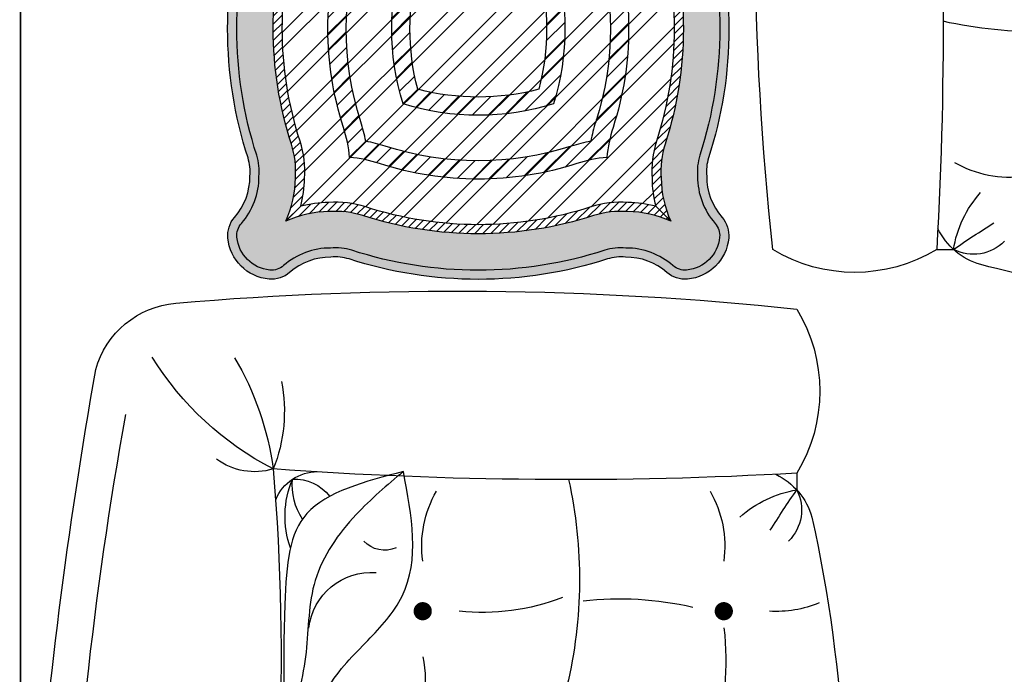
# Model space of a CAD drawing. Units: inches. Extents: x 844 to 2234, y 346 to 1084.
# Tile 63 of 93: x 1843.09 to 1860.31, y 712.91 to 724.36. Entities that reach past the tile are written whole.
import ezdxf

# ---------------------------------------------------------------- set-up
doc = ezdxf.new("R2010")
doc.units = ezdxf.units.IN
doc.header["$MEASUREMENT"] = 0
doc.layers.add('A-WALL', color=7, linetype='Continuous', lineweight=35)
doc.layers.add('furniture', color=8, linetype='Continuous', lineweight=18)
for name, color, linetype in [('RA-AP-01$0$FURN', 3, 'Continuous'), ('RA-AP-01$0$steel', 193, 'Continuous'), ('RA-AP-01$0$WOOD', 64, 'Continuous')]:
    doc.layers.add(name, color=color, linetype=linetype)
pattern_1 = [(45, (0, 1.362436106329781), (-0.0088388347648318, 0.0088388347648318), [])]
pattern_2 = [(45, (0, 1.362436106329781), (-0.0044194173824159, 0.0044194173824159), [])]

# ---------------------------------------------------------------- blocks, each defined once
blk = doc.blocks.new('A$C2FCF5309')
at = {"layer": 'RA-AP-01$0$FURN'}
h = blk.add_hatch(dxfattribs=at)
h.set_pattern_fill('ANSI31', color=256, scale=0.1, style=0)
h.set_pattern_definition(pattern_1)
h.paths.add_polyline_path([(5.038683893313746, -5.169250834004607, -0.1583983521602212), (5.038683893312098, -5.373464580902012, 0.0306258898943267), (5.033304057242972, -5.394827569605182, 0.0306258898948892), (5.01194106853941, -5.40020740567441, -0.1028142994996694), (4.878286182323899, -5.414871334512708), (4.863600873530158, -5.43331743520547, 0.1120482678681049), (5.018059823131753, -5.419248541734471, -0.052642197802937), (5.050972078299936, -5.412495590662115, -0.0526421977994963), (5.057725029371615, -5.379583335496025, 0.1583028414702701), (5.057725029372958, -5.163132079409654, -0.052642197806903), (5.050972078299777, -5.130219824239078, -0.0526421977995126), (5.018059823133679, -5.123466873167369, 0.0215995840215353), (4.988903013548211, -5.115372132362452), (4.975007495303644, -5.132826183367946, -0.0289147572844802), (5.011941068537408, -5.142508009226167, 0.0306258898976746), (5.033304057242868, -5.147887845296027, 0.0306258899022411)])
h.paths.add_polyline_path([(4.975007495303645, -5.132826183367946), (4.988903013548211, -5.115372132362452, 0.1362374241599938), (4.801608567045604, -5.12346687316654, -0.0526421978036853), (4.768696311876971, -5.130219824239102, -0.05264219780204), (4.761943360804856, -5.163132079406747, 0.1583028414743723), (4.761943360806116, -5.379583335498449, -0.0526421977955461), (4.768696311877141, -5.412495590662114, -0.0526421978073986), (4.801608567048022, -5.419248541735437, 0.0454484293938888), (4.863600873530158, -5.43331743520547), (4.878286182323899, -5.414871334512708, -0.0546933379798044), (4.80772732164382, -5.40020740567649, 0.030625889903973), (4.786364332934043, -5.394827569605216, 0.0306258898932853), (4.780984496865101, -5.373464580902791, -0.1583983521638281), (4.780984496864308, -5.169250834000963, 0.03062588989692), (4.786364332933943, -5.147887845296004, 0.0306258898946324), (4.807727321637318, -5.142508009226805, -0.1288932573266927)])
h.paths.add_polyline_path([(4.843422214712861, -5.204945727074827, -0.0783685831716868), (4.924134454130224, -5.196727409635105), (4.939146578618322, -5.177870798323143, 0.1012675676854134), (4.827248748758957, -5.188772261120899, 0.1253648873081696), (4.820394258584192, -5.327034652050361), (4.837127701354095, -5.306015906404253, -0.0981593964869636)], flags=17)
h.paths.add_polyline_path([(4.843422214712824, -5.337769687826355, -0.0311091841722656), (4.837127701354095, -5.306015906404253), (4.820394258584193, -5.32703465205036, 0.0247727657431944), (4.827248748758908, -5.353943153780261, 0.0812754385032542), (4.916962478476905, -5.36629034358622), (4.933684093813825, -5.345286454285511, -0.0876255421014372)], flags=17)
h.paths.add_polyline_path([(4.992419641418037, -5.353943153780226, 0.1506053783834298), (4.992419641417933, -5.188772261120954, 0.0485966419124224), (4.939146578618321, -5.177870798323143), (4.924134454130224, -5.196727409635105, -0.0507799419579301), (4.976246175464031, -5.204945727074882, -0.1296645318906876), (4.97624617546411, -5.337769687826316, -0.0415667119298777), (4.933684093813825, -5.345286454285511), (4.916962478476905, -5.36629034358622, 0.0684915676023693)], flags=17)
h = blk.add_hatch(dxfattribs=at)
h.set_pattern_fill('ANSI31', color=256, scale=0.1, style=0)
h.set_pattern_definition(pattern_1)
h.paths.add_polyline_path([(5.038683893313746, -5.169250834004607, -0.1583983521602212), (5.038683893312098, -5.373464580902012, 0.0306258898943267), (5.033304057242972, -5.394827569605182, 0.0306258898948892), (5.01194106853941, -5.40020740567441, -0.1028142994996694), (4.878286182323899, -5.414871334512708), (4.863600873530158, -5.43331743520547, 0.1120482678681049), (5.018059823131753, -5.419248541734471, -0.052642197802937), (5.050972078299936, -5.412495590662115, -0.0526421977994963), (5.057725029371615, -5.379583335496025, 0.1583028414702701), (5.057725029372958, -5.163132079409654, -0.052642197806903), (5.050972078299777, -5.130219824239078, -0.0526421977995126), (5.018059823133679, -5.123466873167369, 0.0215995840215353), (4.988903013548211, -5.115372132362452), (4.975007495303644, -5.132826183367946, -0.0289147572844802), (5.011941068537408, -5.142508009226167, 0.0306258898976746), (5.033304057242868, -5.147887845296027, 0.0306258899022411)])
h.paths.add_polyline_path([(4.975007495303645, -5.132826183367946), (4.988903013548211, -5.115372132362452, 0.1362374241599938), (4.801608567045604, -5.12346687316654, -0.0526421978036853), (4.768696311876971, -5.130219824239102, -0.05264219780204), (4.761943360804856, -5.163132079406747, 0.1583028414743723), (4.761943360806116, -5.379583335498449, -0.0526421977955461), (4.768696311877141, -5.412495590662114, -0.0526421978073986), (4.801608567048022, -5.419248541735437, 0.0454484293938888), (4.863600873530158, -5.43331743520547), (4.878286182323899, -5.414871334512708, -0.0546933379798044), (4.80772732164382, -5.40020740567649, 0.030625889903973), (4.786364332934043, -5.394827569605216, 0.0306258898932853), (4.780984496865101, -5.373464580902791, -0.1583983521638281), (4.780984496864308, -5.169250834000963, 0.03062588989692), (4.786364332933943, -5.147887845296004, 0.0306258898946324), (4.807727321637318, -5.142508009226805, -0.1288932573266927)])
h.paths.add_polyline_path([(4.843422214712861, -5.204945727074827, -0.0783685831716868), (4.924134454130224, -5.196727409635105), (4.939146578618322, -5.177870798323143, 0.1012675676854134), (4.827248748758957, -5.188772261120899, 0.1253648873081696), (4.820394258584192, -5.327034652050361), (4.837127701354095, -5.306015906404253, -0.0981593964869636)], flags=17)
h.paths.add_polyline_path([(4.843422214712824, -5.337769687826355, -0.0311091841722656), (4.837127701354095, -5.306015906404253), (4.820394258584193, -5.32703465205036, 0.0247727657431944), (4.827248748758908, -5.353943153780261, 0.0812754385032542), (4.916962478476905, -5.36629034358622), (4.933684093813825, -5.345286454285511, -0.0876255421014372)], flags=17)
h.paths.add_polyline_path([(4.992419641418037, -5.353943153780226, 0.1506053783834298), (4.992419641417933, -5.188772261120954, 0.0485966419124224), (4.939146578618321, -5.177870798323143), (4.924134454130224, -5.196727409635105, -0.0507799419579301), (4.976246175464031, -5.204945727074882, -0.1296645318906876), (4.97624617546411, -5.337769687826316, -0.0415667119298777), (4.933684093813825, -5.345286454285511), (4.916962478476905, -5.36629034358622, 0.0684915676023693)], flags=17)
at = {"layer": 'RA-AP-01$0$WOOD'}
h = blk.add_hatch(color=256, dxfattribs=at)
edge = h.paths.add_edge_path()
edge.add_arc((4.683001772622394, -5.026441828662609), 0.0299999999999998, 48.77105092035535, 95.25687599427813)
edge.add_arc((4.684834195088484, -5.046357707450686), 0.0499999999998897, 95.25687599443106, 174.7431240064049)
edge.add_arc((4.664918316300367, -5.044525284985046), 0.0300000000000005, 174.7431240062535, 221.2289490796905)
edge.add_arc((4.591236830209155, -5.109094338216345), 0.0679700159630267, -0.5333070513215148, 41.228949079691915, ccw=False)
edge.add_arc((4.609451302807284, -5.114694777173187), 0.0500000000000008, -17.3556839752095, 5.7020707654044145, ccw=False)
edge.add_arc((5.095208119646659, -5.271357707450659), 0.4603971832811796, 162.0683908477609, 197.9316091523306)
edge.add_arc((4.609451302807533, -5.428020637728902), 0.0500000000000006, -5.702070765320514, 17.355683975293914, ccw=False)
edge.add_arc((4.591236830209412, -5.433621076685779), 0.0679700159630261, -41.228949079600625, 0.5333070514128053, ccw=False)
edge.add_arc((4.664918316300727, -5.498190129916959), 0.0299999999999995, 138.7710509204022, 185.256875994324)
edge.add_arc((4.684834195088642, -5.496357707450695), 0.0499999999997451, 185.2568759946742, 264.74312400432)
edge.add_arc((4.683001772622394, -5.516273586238612), 0.03, 264.743124003969, 311.2289490796446)
edge.add_arc((4.747570825853633, -5.589955072329876), 0.0679700159630271, 89.4666929486321, 131.2289490796457, ccw=False)
edge.add_arc((4.753171264810493, -5.57174059973175), 0.0500000000000015, 72.64431602474701, 95.70207076536133, ccw=False)
edge.add_arc((4.909834195088355, -5.085983782892503), 0.4603971832811774, 252.0683908477147, 287.9316091522845)
edge.add_arc((5.06649712536621, -5.57174059973175), 0.0499999999999999, 84.29792923463953, 107.35568397525361, ccw=False)
edge.add_arc((5.072097564323069, -5.589955072329877), 0.0679700159630274, 48.771050920354185, 90.5333070513679, ccw=False)
edge.add_arc((5.136666617554309, -5.516273586238614), 0.0299999999999997, 228.771050920353, 275.2568759942969)
edge.add_arc((5.134834195088338, -5.496357707450417), 0.0499999999999982, 275.2568759942949, 354.7431240057633)
edge.add_arc((5.154750073876535, -5.498190129916372), 0.0299999999999999, 354.7431240057662, 401.2289490796891)
edge.add_arc((5.228431559967749, -5.433621076685074), 0.0679700159630274, 179.4666929486771, 221.2289490796903, ccw=False)
edge.add_arc((5.210217087369615, -5.428020637728227), 0.0499999999999976, 162.6443160247947, 185.7020707654089, ccw=False)
edge.add_arc((4.724460270530244, -5.271357707450757), 0.4603971832811793, 342.0683908477607, 377.9316091523305)
edge.add_arc((5.210217087369368, -5.114694777172509), 0.0500000000000019, 174.2979292346878, 197.355683975302, ccw=False)
edge.add_arc((5.228431559967489, -5.109094338215639), 0.0679700159630279, 138.7710509203993, 180.5333070514128, ccw=False)
edge.add_arc((5.154750073876174, -5.044525284984457), 0.0300000000000001, 318.771050920401, 365.2568759954636)
edge.add_arc((5.13483419508816, -5.046357707450624), 0.0499999999998349, 5.256875995237118, 84.74312400549572)
edge.add_arc((5.136666617554308, -5.026441828662608), 0.0299999999999994, 84.74312400572185, 131.2289490796446)
edge.add_arc((5.072097564323072, -4.952760342571343), 0.0679700159630261, 269.4666929486298, 311.22894907964354, ccw=False)
edge.add_arc((5.066497125366206, -4.97097481516947), 0.0499999999999992, 252.64431602475162, 275.70207076536565, ccw=False)
edge.add_arc((4.909834195088355, -5.456731632008717), 0.4603971832811764, 72.06839084771546, 107.9316091522853)
edge.add_arc((4.753171264810493, -4.970974815169471), 0.0500000000000016, 264.2979292346387, 287.355683975253, ccw=False)
edge.add_arc((4.747570825853633, -4.952760342571346), 0.0679700159630274, 228.7710509203543, 270.5333070513679, ccw=False)
edge = h.paths.add_edge_path(flags=16)
edge.add_arc((4.683001772622395, -5.026441828662608), 0.019999999999999, 48.7710509203555, 95.2568759942793)
edge.add_arc((4.684834195088469, -5.046357707450671), 0.0399999999998731, 95.2568759944489, 174.7431240064248)
edge.add_arc((4.664918316300404, -5.044525284985035), 0.020000000000036, 174.7431240062186, 221.2289490796461)
edge.add_arc((4.591236830209151, -5.109094338216346), 0.0779700159630296, -0.13764630038667747, 41.228949079689585, ccw=False)
edge.add_arc((4.609451302807307, -5.11469477717304), 0.060000000000024, -17.406127045137907, 5.176192161068002, ccw=False)
edge.add_arc((5.09520811964665, -5.271357707450659), 0.4503971832811708, 162.0623235129628, 197.9376764869162)
edge.add_arc((4.609451302807532, -5.428020637728943), 0.0599999999999982, -5.176192160466428, 17.406127046715312, ccw=False)
edge.add_arc((4.591236830209414, -5.433621076685778), 0.0779700159630257, -41.2289490796029, 0.13764630095249686, ccw=False)
edge.add_arc((4.664918316300731, -5.498190129916961), 0.0200000000000047, 138.7710509204103, 185.2568759943212)
edge.add_arc((4.684834195088606, -5.496357707450731), 0.0399999999997066, 185.2568759947174, 264.7431240043665)
edge.add_arc((4.683001772622369, -5.516273586238541), 0.020000000000069, 264.7431240038842, 311.2289490795622)
edge.add_arc((4.747570825853635, -5.589955072329884), 0.0779700159630344, 89.8623536987642, 131.2289490796432, ccw=False)
edge.add_arc((4.753171264810603, -5.571740599731771), 0.0599999999999895, 72.5938729544394, 95.1761921602253, ccw=False)
edge.add_arc((4.909834195088365, -5.085983782892505), 0.4503971832811724, 252.0623235129989, 287.9376764870498)
edge.add_arc((5.066497125366216, -5.571740599731755), 0.0600000000000047, 84.8238078399923, 107.40612704528041, ccw=False)
edge.add_arc((5.072097564322998, -5.589955072329853), 0.077970015963056, 48.771050920303594, 90.13764630126451, ccw=False)
edge.add_arc((5.136666617554307, -5.516273586238622), 0.0199999999999931, 228.771050920344, 275.2568759943037)
edge.add_arc((5.134834195088338, -5.496357707450416), 0.0400000000000004, 275.2568759942928, 354.7431240057607)
edge.add_arc((5.154750073876533, -5.498190129916375), 0.0200000000000037, 354.7431240057783, 401.2289490796939)
edge.add_arc((5.228431559967745, -5.433621076685076), 0.0779700159630239, 179.8623536995147, 221.2289490796908, ccw=False)
edge.add_arc((5.210217087369586, -5.428020637728345), 0.0600000000000054, 162.5938729554486, 185.1761921609759, ccw=False)
edge.add_arc((4.724460270530243, -5.271357707450766), 0.4503971832811826, 342.0623235128896, 377.937676486982)
edge.add_arc((5.210217087369347, -5.114694777172486), 0.0599999999999777, 174.8238078387611, 197.4061270462219, ccw=False)
edge.add_arc((5.228431559967523, -5.109094338215542), 0.0779700159629885, 138.7710509204687, 180.1376463004423, ccw=False)
edge.add_arc((5.154750073876175, -5.044525284984459), 0.0199999999999989, 318.771050920406, 365.2568759954698)
edge.add_arc((5.134834195088138, -5.046357707450646), 0.0399999999998586, 5.256875995208452, 84.74312400546732)
edge.add_arc((5.136666617554292, -5.02644182866256), 0.0199999999999529, 84.74312400577769, 131.2289490797025)
edge.add_arc((5.072097564323069, -4.952760342571338), 0.077970015963032, 269.86235369901414, 311.2289490796421, ccw=False)
edge.add_arc((5.06649712536618, -4.97097481516946), 0.0600000000000007, 252.5938729548277, 275.17619216047467, ccw=False)
edge.add_arc((4.909834195088353, -5.456731632008716), 0.4503971832811739, 72.06232351293887, 107.9376764867365)
edge.add_arc((4.753171264810429, -4.970974815169467), 0.0599999999999991, 264.82380783985815, 287.40612704769893, ccw=False)
edge.add_arc((4.747570825853681, -4.952760342571361), 0.0779700159630467, 228.7710509203206, 270.13764630113724, ccw=False)
h = blk.add_hatch(color=256, dxfattribs=at)
edge = h.paths.add_edge_path()
edge.add_arc((4.683001772622395, -5.026441828662608), 0.019999999999999, 48.7710509203555, 95.2568759942793)
edge.add_arc((4.684834195088469, -5.046357707450671), 0.0399999999998731, 95.2568759944489, 174.7431240064248)
edge.add_arc((4.664918316300404, -5.044525284985035), 0.020000000000036, 174.7431240062186, 221.2289490796461)
edge.add_arc((4.591236830209151, -5.109094338216346), 0.0779700159630296, -0.13764630038667747, 41.228949079689585, ccw=False)
edge.add_arc((4.609451302807307, -5.11469477717304), 0.060000000000024, -17.406127045137907, 5.176192161068002, ccw=False)
edge.add_arc((5.09520811964665, -5.271357707450659), 0.4503971832811708, 162.0623235129628, 197.9376764869162)
edge.add_arc((4.609451302807532, -5.428020637728943), 0.0599999999999982, -5.176192160466428, 17.406127046715312, ccw=False)
edge.add_arc((4.591236830209414, -5.433621076685778), 0.0779700159630257, -41.2289490796029, 0.13764630095249686, ccw=False)
edge.add_arc((4.664918316300731, -5.498190129916961), 0.0200000000000047, 138.7710509204103, 185.2568759943212)
edge.add_arc((4.684834195088606, -5.496357707450731), 0.0399999999997066, 185.2568759947174, 264.7431240043665)
edge.add_arc((4.683001772622369, -5.516273586238541), 0.020000000000069, 264.7431240038842, 311.2289490795622)
edge.add_arc((4.747570825853635, -5.589955072329884), 0.0779700159630344, 89.8623536987642, 131.2289490796432, ccw=False)
edge.add_arc((4.753171264810603, -5.571740599731771), 0.0599999999999895, 72.5938729544394, 95.1761921602253, ccw=False)
edge.add_arc((4.909834195088365, -5.085983782892505), 0.4503971832811724, 252.0623235129989, 287.9376764870498)
edge.add_arc((5.066497125366216, -5.571740599731755), 0.0600000000000047, 84.8238078399923, 107.40612704528041, ccw=False)
edge.add_arc((5.072097564322998, -5.589955072329853), 0.077970015963056, 48.771050920303594, 90.13764630126451, ccw=False)
edge.add_arc((5.136666617554307, -5.516273586238622), 0.0199999999999931, 228.771050920344, 275.2568759943037)
edge.add_arc((5.134834195088338, -5.496357707450416), 0.0400000000000004, 275.2568759942928, 354.7431240057607)
edge.add_arc((5.154750073876533, -5.498190129916375), 0.0200000000000037, 354.7431240057783, 401.2289490796939)
edge.add_arc((5.228431559967745, -5.433621076685076), 0.0779700159630239, 179.8623536995147, 221.2289490796908, ccw=False)
edge.add_arc((5.210217087369586, -5.428020637728345), 0.0600000000000054, 162.5938729554486, 185.1761921609759, ccw=False)
edge.add_arc((4.724460270530243, -5.271357707450766), 0.4503971832811826, 342.0623235128896, 377.937676486982)
edge.add_arc((5.210217087369347, -5.114694777172486), 0.0599999999999777, 174.8238078387611, 197.4061270462219, ccw=False)
edge.add_arc((5.228431559967523, -5.109094338215542), 0.0779700159629885, 138.7710509204687, 180.1376463004423, ccw=False)
edge.add_arc((5.154750073876175, -5.044525284984459), 0.0199999999999989, 318.771050920406, 365.2568759954698)
edge.add_arc((5.134834195088138, -5.046357707450646), 0.0399999999998586, 5.256875995208452, 84.74312400546732)
edge.add_arc((5.136666617554292, -5.02644182866256), 0.0199999999999529, 84.74312400577769, 131.2289490797025)
edge.add_arc((5.072097564323069, -4.952760342571338), 0.077970015963032, 269.86235369901414, 311.2289490796421, ccw=False)
edge.add_arc((5.06649712536618, -4.97097481516946), 0.0600000000000007, 252.5938729548277, 275.17619216047467, ccw=False)
edge.add_arc((4.909834195088353, -5.456731632008716), 0.4503971832811739, 72.06232351293887, 107.9376764867365)
edge.add_arc((4.753171264810429, -4.970974815169467), 0.0599999999999991, 264.82380783985815, 287.40612704769893, ccw=False)
edge.add_arc((4.747570825853681, -4.952760342571361), 0.0779700159630467, 228.7710509203206, 270.13764630113724, ccw=False)
edge = h.paths.add_edge_path(flags=16)
edge.add_arc((4.591236830209151, -5.109094338216348), 0.1179700159630308, 0.7417751874182841, 24.563326950263672, ccw=False)
edge.add_arc((4.609451302807302, -5.114694777173093), 0.100000000000012, -17.52836504564658, 4.087328884225087, ccw=False)
edge.add_arc((5.095208119646651, -5.271357707450657), 0.4103971832811724, 162.0403002448777, 197.9596997550675)
edge.add_arc((4.60945130280753, -5.428020637728918), 0.1000000000000027, -4.087328883827581, 17.528365046291924, ccw=False)
edge.add_arc((4.591236830209414, -5.433621076685779), 0.1179700159630246, 335.43667305041845, 359.2582248129738, ccw=False)
edge.add_arc((4.747570825853596, -5.589955072329891), 0.117970015963042, 90.7417751868461, 114.5633269496104, ccw=False)
edge.add_arc((4.753171264810559, -5.571740599731767), 0.0999999999999976, 72.47163495370341, 94.0873288836737, ccw=False)
edge.add_arc((4.909834195088367, -5.085983782892503), 0.4103971832811735, 252.0403002449999, 287.9596997551833)
edge.add_arc((5.066497125366205, -5.571740599731755), 0.1000000000000057, 85.91267111645209, 107.5283650455624, ccw=False)
edge.add_arc((5.072097564322985, -5.58995507232986), 0.117970015963046, 65.4366730497672, 89.25822481317113, ccw=False)
edge.add_arc((5.22843155996773, -5.433621076684992), 0.1179700159630096, 180.7417751873964, 204.5633269502712, ccw=False)
edge.add_arc((5.210217087369591, -5.428020637728301), 0.0999999999999969, 162.4716349546276, 184.0873288841682, ccw=False)
edge.add_arc((4.724460270530243, -5.271357707450766), 0.4103971832811825, 342.0403002448147, 377.9596997550345)
edge.add_arc((5.210217087369347, -5.114694777172489), 0.0999999999999796, 175.9126711156995, 197.5283650464392, ccw=False)
edge.add_arc((5.228431559967512, -5.109094338215525), 0.1179700159630019, 155.4366730502992, 179.2582248126247, ccw=False)
edge.add_arc((5.072097564323172, -4.952760342571314), 0.1179700159630537, 270.74177518697286, 294.56332694975765, ccw=False)
edge.add_arc((5.066497125366189, -4.970974815169462), 0.1000000000000017, 252.471634954247, 274.0873288838353, ccw=False)
edge.add_arc((4.909834195088353, -5.456731632008716), 0.4103971832811758, 72.04030024486342, 107.9596997549354)
edge.add_arc((4.75317126481046, -4.970974815169467), 0.1000000000000041, 265.91267111635307, 287.5283650466103, ccw=False)
edge.add_arc((4.747570825853629, -4.952760342571342), 0.1179700159630538, 245.43667304992562, 269.2582248131125, ccw=False)
h = blk.add_hatch(dxfattribs=at)
h.set_pattern_fill('ANSI31', color=256, scale=0.05, style=0)
h.set_pattern_definition(pattern_2)
h.paths.add_polyline_path([(5.105336294329346, -5.394854099602528, 0.0940138826956367), (5.100476366643778, -5.435568764288975, 0.0606271852326483), (5.104678567100611, -5.466202079462671, 0.0606271852344644), (5.074045251925975, -5.46199987900586, 0.0940138827021426), (5.033330587236848, -5.466859806692645, -0.1305325492494615), (4.828072633169377, -5.477944178050054), (4.821119726105699, -5.486677669841435, 0.1336226599878005), (5.036379334063467, -5.476383803188216, -0.0945969211935747), (5.073624810952389, -5.471994942692536, -0.1043170707892296), (5.121137550891356, -5.48266106325342, -0.1043170707868944), (5.110471430330457, -5.435148323315565, -0.0945969211952573), (5.114860290825935, -5.397902846425963, 0.1580239521433527), (5.114860290826324, -5.144812568476775, -0.0945969212010491), (5.110471430330247, -5.10756709158498, -0.1043170707844371), (5.121137550890657, -5.060054351648168, -0.104317070786514), (5.073624810952866, -5.070720472208642, -0.0945969211958523), (5.036379334063063, -5.066331611712874, 0.1580239521426795), (4.783289056114906, -5.066331611712465, -0.0945969211985319), (4.746043579224103, -5.070720472208672, -0.1043170707882665), (4.698530839285552, -5.060054351647925, -0.1043170707867205), (4.709196959846443, -5.10756709158571, -0.094596921196788), (4.704808099350826, -5.144812568475902, 0.1580239521433127), (4.704808099350699, -5.397902846425022, -0.094596921197841), (4.709196959846712, -5.435148323315576, -0.1043170707855109), (4.698530839286393, -5.482661063252921, -0.1043170707864168), (4.746043579224162, -5.471994942692571, -0.0945969211977586), (4.783289056114671, -5.476383803188671, 0.0238966994662183), (4.821119726105699, -5.486677669841435), (4.828072633169378, -5.477944178050054, -0.0269814195959459), (4.786337802940177, -5.466859806692736, 0.0940138827039629), (4.745623138250268, -5.461999879005895, 0.0606271852320776), (4.714989823076826, -5.466202079462476, 0.0606271852304618), (4.719192023533341, -5.435568764289856, 0.0940138826917763), (4.714332095848404, -5.394854099604977, -0.1580706864542086), (4.714332095846561, -5.147861315302034, 0.0940138827032017), (4.719192023533127, -5.107146650612438, 0.0606271852329446), (4.714989823076289, -5.076513335438588, 0.0606271852340035), (4.745623138250698, -5.08071553589536, 0.0940138827025969), (4.786337802940015, -5.075855608208526, -0.1580706864508517), (5.033330587237968, -5.075855608208939, 0.0940138827009578), (5.074045251926627, -5.080715535895319, 0.0606271852322557), (5.104678567100159, -5.076513335438697, 0.0606271852308743), (5.100476366643561, -5.107146650611519, 0.0940138827178109), (5.105336294331983, -5.147861315307182, -0.1580706864490946)])
h = blk.add_hatch(dxfattribs=at)
h.set_pattern_fill('ANSI31', color=256, scale=0.05, style=0)
h.set_pattern_definition(pattern_2)
h.paths.add_polyline_path([(5.105336294329346, -5.394854099602528, 0.0940138826956367), (5.100476366643778, -5.435568764288975, 0.0606271852326483), (5.104678567100611, -5.466202079462671, 0.0606271852344644), (5.074045251925975, -5.46199987900586, 0.0940138827021426), (5.033330587236848, -5.466859806692645, -0.1305325492494615), (4.828072633169377, -5.477944178050054), (4.821119726105699, -5.486677669841435, 0.1336226599878005), (5.036379334063467, -5.476383803188216, -0.0945969211935747), (5.073624810952389, -5.471994942692536, -0.1043170707892296), (5.121137550891356, -5.48266106325342, -0.1043170707868944), (5.110471430330457, -5.435148323315565, -0.0945969211952573), (5.114860290825935, -5.397902846425963, 0.1580239521433527), (5.114860290826324, -5.144812568476775, -0.0945969212010491), (5.110471430330247, -5.10756709158498, -0.1043170707844371), (5.121137550890657, -5.060054351648168, -0.104317070786514), (5.073624810952866, -5.070720472208642, -0.0945969211958523), (5.036379334063063, -5.066331611712874, 0.1580239521426795), (4.783289056114906, -5.066331611712465, -0.0945969211985319), (4.746043579224103, -5.070720472208672, -0.1043170707882665), (4.698530839285552, -5.060054351647925, -0.1043170707867205), (4.709196959846443, -5.10756709158571, -0.094596921196788), (4.704808099350826, -5.144812568475902, 0.1580239521433127), (4.704808099350699, -5.397902846425022, -0.094596921197841), (4.709196959846712, -5.435148323315576, -0.1043170707855109), (4.698530839286393, -5.482661063252921, -0.1043170707864168), (4.746043579224162, -5.471994942692571, -0.0945969211977586), (4.783289056114671, -5.476383803188671, 0.0238966994662183), (4.821119726105699, -5.486677669841435), (4.828072633169378, -5.477944178050054, -0.0269814195959459), (4.786337802940177, -5.466859806692736, 0.0940138827039629), (4.745623138250268, -5.461999879005895, 0.0606271852320776), (4.714989823076826, -5.466202079462476, 0.0606271852304618), (4.719192023533341, -5.435568764289856, 0.0940138826917763), (4.714332095848404, -5.394854099604977, -0.1580706864542086), (4.714332095846561, -5.147861315302034, 0.0940138827032017), (4.719192023533127, -5.107146650612438, 0.0606271852329446), (4.714989823076289, -5.076513335438588, 0.0606271852340035), (4.745623138250698, -5.08071553589536, 0.0940138827025969), (4.786337802940015, -5.075855608208526, -0.1580706864508517), (5.033330587237968, -5.075855608208939, 0.0940138827009578), (5.074045251926627, -5.080715535895319, 0.0606271852322557), (5.104678567100159, -5.076513335438697, 0.0606271852308743), (5.100476366643561, -5.107146650611519, 0.0940138827178109), (5.105336294331983, -5.147861315307182, -0.1580706864490946)])
h = blk.add_hatch(dxfattribs=at)
h.set_pattern_fill('ANSI32,_I', color=256, scale=0.1, style=2)
h.set_pattern_definition([(45, (0, 0), (-0.0265165042944955, 0.0265165042944955), []), (45, (0.0176776695, 0), (-0.0265165042944955, 0.0265165042944955), [])])
h.paths.add_polyline_path([(4.843422214712824, -5.337769687826354, 0.1296645318905289), (4.97624617546411, -5.337769687826316, 0.1296645318906876), (4.976246175464032, -5.204945727074882, 0.129664531890418), (4.843422214712861, -5.204945727074827, 0.129664531890765)], flags=0)
h.paths.add_polyline_path([(5.039131224122924, -5.170637849998464, -0.0326520429852175), (5.033304057242868, -5.147887845296027, -0.0326520429894721), (5.010554052537512, -5.142060678415043, 0.1561383235202698), (4.809114337641437, -5.142060678414318, -0.0326520429925972), (4.786364332933944, -5.147887845296004, -0.0326520429914489), (4.780537166052582, -5.170637850002729, 0.1561383235189577), (4.780537166052134, -5.37207756489719, -0.0326520429934175), (4.786364332934042, -5.394827569605215, -0.0326520429823496), (4.809114337634529, -5.400654736484653, 0.156138323524066), (5.010554052535268, -5.400654736486903, -0.032652042992888), (5.033304057242972, -5.394827569605183, -0.0326520429928733), (5.039131224124712, -5.372077564897496, 0.1561383235226786)], flags=0)
h.paths.add_polyline_path([(4.992419641418037, -5.353943153780226, -0.1506053783832862), (4.827248748758909, -5.353943153780261, -0.1506053783835069), (4.827248748758957, -5.188772261120899, -0.1506053783831346), (4.992419641417933, -5.188772261120954, -0.1506053783834298)], flags=0)
h.paths.add_polyline_path([(4.976246175464111, -5.337769687826316, -0.1296645318905298), (4.843422214712824, -5.337769687826354, -0.129664531890765), (4.843422214712862, -5.204945727074827, -0.1296645318904162), (4.976246175464031, -5.204945727074882, -0.1296645318906876)], flags=0)
h.paths.add_polyline_path([(5.105721254232479, -5.149054940982025, -0.0968902512052664), (5.100476366643561, -5.107146650611519, -0.0606271852308743), (5.104678567100159, -5.076513335438697, -0.0606271852322574), (5.074045251926626, -5.080715535895319, -0.0968902512197216), (5.032136961550132, -5.075470648304253, 0.1564657949319774), (4.787531428625239, -5.075470648304682, -0.0968902512150626), (4.745623138250699, -5.08071553589536, -0.060627185234009), (4.714989823076288, -5.076513335438587, -0.0606271852329501), (4.719192023533127, -5.10714665061244, -0.0968902512185585), (4.713947135942331, -5.149054940988458, 0.1564657949285579), (4.713947135940853, -5.393660473908259, -0.0968902512319826), (4.71919202353334, -5.435568764289873, -0.0606271852304288), (4.714989823076825, -5.466202079462476, -0.0606271852320811), (4.745623138250269, -5.461999879005895, -0.0968902512162649), (4.787531428625332, -5.467244766596559, 0.1564657949327057), (5.032136961551311, -5.46724476659659, -0.0968902512153659), (5.074045251925975, -5.46199987900586, -0.0606271852344627), (5.10467856710061, -5.466202079462671, -0.0606271852326483), (5.100476366643777, -5.435568764288975, -0.0968902512258216), (5.105721254235559, -5.393660473909953, 0.1564657949340142)])
h.paths.add_polyline_path([(5.057725029371625, -5.379583335495999, 0.0526421977995391), (5.050972078299936, -5.412495590662114, 0.0526421978029782), (5.018059823131728, -5.419248541734479, -0.1583028414681072), (4.801608567048168, -5.419248541735485, 0.0526421978076402), (4.76869631187714, -5.412495590662113, 0.0526421977956189), (4.761943360806101, -5.379583335498404, -0.1583028414743129), (4.761943360804846, -5.163132079406778, 0.0526421978020944), (4.768696311876972, -5.130219824239101, 0.0526421978033651), (4.80160856704541, -5.123466873166602, -0.1583028414716875), (5.018059823133628, -5.123466873167353, 0.0526421977995944), (5.050972078299776, -5.130219824239078, 0.0526421978070423), (5.057725029372986, -5.163132079409739, -0.1583028414701848)], flags=16)
h.paths.add_polyline_path([(5.038683893312112, -5.373464580901968, 0.0306258898943915), (5.033304057242972, -5.394827569605182, 0.0306258898948892), (5.01194106853941, -5.40020740567441, -0.1583983521587032), (4.807727321643864, -5.400207405676503, 0.0306258899040366), (4.786364332934043, -5.394827569605215, 0.0306258898931986), (4.780984496865119, -5.37346458090285, -0.1583983521638542), (4.7809844968643, -5.169250834000989, 0.0306258898969596), (4.786364332933945, -5.147887845296004, 0.0306258898946195), (4.807727321637311, -5.142508009226808, -0.1583983521623412), (5.011941068537318, -5.142508009226139, 0.030625889897807), (5.033304057242868, -5.147887845296028, 0.0306258899020632), (5.038683893313706, -5.169250834004486, -0.1583983521602835)], flags=0)
for p, q in [((4.714989823076289, -5.076513335438588), (4.698530839285552, -5.060054351647925)), ((4.714989823076289, -5.076513335438588), (4.698530839285552, -5.060054351647925)), ((5.104678567100159, -5.076513335438697), (5.121137550890656, -5.060054351648169)), ((5.104678567100159, -5.076513335438697), (5.121137550890656, -5.060054351648169)), ((5.10467856710061, -5.466202079462671), (5.121137550891355, -5.482661063253419)), ((5.10467856710061, -5.466202079462671), (5.121137550891355, -5.482661063253419))]:
    blk.add_line(p, q, dxfattribs=at)
for points in [[(4.702773858784635, -5.003879368495489, 0.2056608120285223), (4.680253138923443, -4.996568010480312, 0.3614336704708569), (4.635044498118043, -5.041776651286372, 0.2056608120263112), (4.642355856133262, -5.064297371147306, -0.1842662638101064), (4.65920390179375, -5.10972699154053, -0.1009492694051416), (4.657174869772992, -5.129609908955028, 0.1577727036674954), (4.657174869773219, -5.41310550594699, -0.1009492694051416), (4.659203901794006, -5.432988423361486, -0.1842662638101064), (4.64235585613359, -5.478418043754737, 0.2056608120285221), (4.635044498118431, -5.500938763615934, 0.3614336704593693), (4.680253138922529, -5.546147404420826, 0.2056608120364936), (4.702773858784635, -5.538836046405732, -0.1842662638101064), (4.748203479177874, -5.52198800074528, -0.1009492694051415), (4.768086396592371, -5.524017032766053, 0.1577727036674954), (5.051581993584332, -5.524017032766055, -0.1009492694051416), (5.071464910998829, -5.521988000745282, -0.1842662638101064), (5.116894531392067, -5.538836046405734, 0.2056608120286145), (5.13941525125327, -5.546147404420911, 0.3614336704683636), (5.184623892058835, -5.500938763615299, 0.2056608120285223), (5.177312534043641, -5.478418043754112, -0.1842662638101063), (5.160464488383153, -5.432988423360887, -0.1009492694051416), (5.162493520403909, -5.41310550594639, 0.1577727036674954), (5.162493520403684, -5.129609908954428, -0.1009492694051416), (5.160464488382894, -5.109726991539933, -0.1842662638101064), (5.17731253404331, -5.064297371146681, 0.2056608120337072), (5.184623892058415, -5.041776651284888, 0.3614336704623863), (5.139415251253259, -4.99656801048031, 0.2056608120285223), (5.116894531392067, -5.003879368495487, -0.1842662638101064), (5.071464910998829, -5.020727414155937, -0.1009492694051416), (5.051581993584332, -5.018698382135166, 0.1577727036674956), (4.768086396592371, -5.018698382135168, -0.1009492694051416), (4.748203479177874, -5.020727414155941, -0.1842662638101064)], [(4.702773858784635, -5.003879368495489, 0.2056608120285223), (4.680253138923443, -4.996568010480312, 0.3614336704708569), (4.635044498118043, -5.041776651286372, 0.2056608120263112), (4.642355856133262, -5.064297371147306, -0.1842662638101064), (4.65920390179375, -5.10972699154053, -0.1009492694051416), (4.657174869772992, -5.129609908955028, 0.1577727036674954), (4.657174869773219, -5.41310550594699, -0.1009492694051416), (4.659203901794006, -5.432988423361486, -0.1842662638101064), (4.64235585613359, -5.478418043754737, 0.2056608120285221), (4.635044498118431, -5.500938763615934, 0.3614336704593693), (4.680253138922529, -5.546147404420826, 0.2056608120364936), (4.702773858784635, -5.538836046405732, -0.1842662638101064), (4.748203479177874, -5.52198800074528, -0.1009492694051415), (4.768086396592371, -5.524017032766053, 0.1577727036674954), (5.051581993584332, -5.524017032766055, -0.1009492694051416), (5.071464910998829, -5.521988000745282, -0.1842662638101064), (5.116894531392067, -5.538836046405734, 0.2056608120286145), (5.13941525125327, -5.546147404420911, 0.3614336704683636), (5.184623892058835, -5.500938763615299, 0.2056608120285223), (5.177312534043641, -5.478418043754112, -0.1842662638101063), (5.160464488383153, -5.432988423360887, -0.1009492694051416), (5.162493520403909, -5.41310550594639, 0.1577727036674954), (5.162493520403684, -5.129609908954428, -0.1009492694051416), (5.160464488382894, -5.109726991539933, -0.1842662638101064), (5.17731253404331, -5.064297371146681, 0.2056608120337072), (5.184623892058415, -5.041776651284888, 0.3614336704623863), (5.139415251253259, -4.99656801048031, 0.2056608120285223), (5.116894531392067, -5.003879368495487, -0.1842662638101064), (5.071464910998829, -5.020727414155937, -0.1009492694051416), (5.051581993584332, -5.018698382135166, 0.1577727036674956), (4.768086396592371, -5.018698382135168, -0.1009492694051416), (4.748203479177874, -5.020727414155941, -0.1842662638101064)], [(4.696183163397222, -5.011400188551196, 0.2056608120285295), (4.681169350156427, -5.006525949874411, 0.3614336704708588), (4.645002437512154, -5.042692862519237, 0.2056608120262659), (4.649876676188964, -5.057706675759887, -0.182481815856965), (4.669206621172843, -5.109281651732388, -0.0988540857970112), (4.666703803477437, -5.13264334722805, 0.1578269695851905), (4.666703803477144, -5.410072067672365, -0.0988540858013112), (4.6692066211731, -5.433433763168966, -0.1824818158591246), (4.649876676189301, -5.485008739142145, 0.2056608120284717), (4.64500243751253, -5.500022552382944, 0.3614336704593821), (4.681169350155757, -5.536189465026749, 0.2056608120365057), (4.696183163397221, -5.531315226350026, -0.1824818158605826), (4.747758139370833, -5.51198528136619, -0.0988540857951607), (4.771119834866025, -5.514488099061806, 0.1578269695856264), (5.04854855531107, -5.514488099061688, -0.0988540857929677), (5.071910250805761, -5.511985281366138, -0.1824818158609529), (5.123485226779481, -5.531315226350027, 0.2056608120286893), (5.138499040020282, -5.536189465026812, 0.3614336704683556), (5.174665952664737, -5.500022552382323, 0.2056608120284882), (5.169791713987938, -5.485008739141532, -0.1824818158574124), (5.150461769004059, -5.4334337631689, -0.0988540857940221), (5.152964586699289, -5.410072067673927, 0.1578269695858123), (5.1529645866996, -5.132643347228565, -0.0988540858025403), (5.150461769003872, -5.109281651731659, -0.1824818158565006), (5.169791713987599, -5.057706675759273, 0.2056608120337192), (5.174665952664335, -5.042692862518078, 0.3614336704623903), (5.138499040020236, -5.006525949874406, 0.2056608120285323), (5.123485226779481, -5.011400188551195, -0.1824818158594503), (5.071910250806212, -5.03073013353503, -0.09885408579455), (5.048548555311143, -5.028227315839558, 0.1578269695844942), (4.771119834867991, -5.028227315838772, -0.0988540858042156), (4.747758139370745, -5.030730133535067, -0.1824818158603032)], [(4.696183163397222, -5.011400188551196, 0.2056608120285295), (4.681169350156427, -5.006525949874411, 0.3614336704708588), (4.645002437512154, -5.042692862519237, 0.2056608120262659), (4.649876676188964, -5.057706675759887, -0.182481815856965), (4.669206621172843, -5.109281651732388, -0.0988540857970112), (4.666703803477437, -5.13264334722805, 0.1578269695851905), (4.666703803477144, -5.410072067672365, -0.0988540858013112), (4.6692066211731, -5.433433763168966, -0.1824818158591246), (4.649876676189301, -5.485008739142145, 0.2056608120284717), (4.64500243751253, -5.500022552382944, 0.3614336704593821), (4.681169350155757, -5.536189465026749, 0.2056608120365057), (4.696183163397221, -5.531315226350026, -0.1824818158605826), (4.747758139370833, -5.51198528136619, -0.0988540857951607), (4.771119834866025, -5.514488099061806, 0.1578269695856264), (5.04854855531107, -5.514488099061688, -0.0988540857929677), (5.071910250805761, -5.511985281366138, -0.1824818158609529), (5.123485226779481, -5.531315226350027, 0.2056608120286893), (5.138499040020282, -5.536189465026812, 0.3614336704683556), (5.174665952664737, -5.500022552382323, 0.2056608120284882), (5.169791713987938, -5.485008739141532, -0.1824818158574124), (5.150461769004059, -5.4334337631689, -0.0988540857940221), (5.152964586699289, -5.410072067673927, 0.1578269695858123), (5.1529645866996, -5.132643347228565, -0.0988540858025403), (5.150461769003872, -5.109281651731659, -0.1824818158565006), (5.169791713987599, -5.057706675759273, 0.2056608120337192), (5.174665952664335, -5.042692862518078, 0.3614336704623903), (5.138499040020236, -5.006525949874406, 0.2056608120285323), (5.123485226779481, -5.011400188551195, -0.1824818158594503), (5.071910250806212, -5.03073013353503, -0.09885408579455), (5.048548555311143, -5.028227315839558, 0.1578269695844942), (4.771119834867991, -5.028227315838772, -0.0988540858042156), (4.747758139370745, -5.030730133535067, -0.1824818158603032)], [(4.698530839285552, -5.060054351647925, -0.1043170707867612), (4.709196959846444, -5.107567091585729, -0.0945969211969405), (4.704808099350802, -5.144812568475978, 0.1580239521432241), (4.704808099350681, -5.397902846424963, -0.0945969211980322), (4.709196959846711, -5.43514832331559, -0.104317070785482), (4.698530839286393, -5.482661063252921, -0.1043170707864036), (4.746043579224155, -5.471994942692571, -0.094596921197375), (4.78328905611452, -5.476383803188623, 0.1580239521431959), (5.036379334063463, -5.476383803188218, -0.0945969211935888), (5.07362481095239, -5.471994942692536, -0.1043170707892253), (5.121137550891355, -5.482661063253419, -0.1043170707868921), (5.110471430330457, -5.435148323315565, -0.0945969211954828), (5.114860290825962, -5.397902846425878, 0.158023952143358), (5.114860290826295, -5.144812568476682, -0.0945969212007617), (5.110471430330247, -5.107567091584995, -0.1043170707844689), (5.121137550890656, -5.060054351648169, -0.1043170707864946), (5.073624810952874, -5.070720472208642, -0.0945969211956941), (5.036379334063131, -5.066331611712896, 0.1580239521426976), (4.783289056114946, -5.066331611712452, -0.0945969211986379), (4.746043579224103, -5.070720472208672, -0.1043170707882684)], [(4.698530839285552, -5.060054351647925, -0.1043170707867612), (4.709196959846444, -5.107567091585729, -0.0945969211969405), (4.704808099350802, -5.144812568475978, 0.1580239521432241), (4.704808099350681, -5.397902846424963, -0.0945969211980322), (4.709196959846711, -5.43514832331559, -0.104317070785482), (4.698530839286393, -5.482661063252921, -0.1043170707864036), (4.746043579224155, -5.471994942692571, -0.094596921197375), (4.78328905611452, -5.476383803188623, 0.1580239521431959), (5.036379334063463, -5.476383803188218, -0.0945969211935888), (5.07362481095239, -5.471994942692536, -0.1043170707892253), (5.121137550891355, -5.482661063253419, -0.1043170707868921), (5.110471430330457, -5.435148323315565, -0.0945969211954828), (5.114860290825962, -5.397902846425878, 0.158023952143358), (5.114860290826295, -5.144812568476682, -0.0945969212007617), (5.110471430330247, -5.107567091584995, -0.1043170707844689), (5.121137550890656, -5.060054351648169, -0.1043170707864946), (5.073624810952874, -5.070720472208642, -0.0945969211956941), (5.036379334063131, -5.066331611712896, 0.1580239521426976), (4.783289056114946, -5.066331611712452, -0.0945969211986379), (4.746043579224103, -5.070720472208672, -0.1043170707882684)], [(4.714989823076289, -5.076513335438588, -0.0606271852329464), (4.719192023533127, -5.107146650612439, -0.0940138827030756), (4.714332095846578, -5.147861315301983, 0.1580706864542707), (4.714332095848417, -5.394854099605018, -0.0940138826916965), (4.719192023533341, -5.435568764289864, -0.0606271852304462), (4.714989823076826, -5.466202079462476, -0.0606271852320585), (4.745623138250258, -5.461999879005895, -0.0940138827037036), (4.786337802940059, -5.466859806692699, 0.1580706864500221), (5.033330587236783, -5.466859806692666, -0.0940138827023111), (5.074045251925979, -5.46199987900586, -0.060627185234454), (5.10467856710061, -5.466202079462671, -0.0606271852326709), (5.100476366643777, -5.435568764288963, -0.0940138826958686), (5.105336294329379, -5.394854099602421, 0.1580706864489859), (5.105336294331999, -5.147861315307237, -0.0940138827179432), (5.100476366643561, -5.107146650611518, -0.0606271852308726), (5.104678567100159, -5.076513335438697, -0.0606271852322592), (5.074045251926625, -5.080715535895319, -0.094013882701022), (5.03333058723794, -5.075855608208931, 0.1580706864508015), (4.786337802940061, -5.075855608208511, -0.0940138827027143), (4.745623138250695, -5.08071553589536, -0.0606271852339983)], [(4.714989823076289, -5.076513335438588, -0.0606271852329464), (4.719192023533127, -5.107146650612439, -0.0940138827030756), (4.714332095846578, -5.147861315301983, 0.1580706864542707), (4.714332095848417, -5.394854099605018, -0.0940138826916965), (4.719192023533341, -5.435568764289864, -0.0606271852304462), (4.714989823076826, -5.466202079462476, -0.0606271852320585), (4.745623138250258, -5.461999879005895, -0.0940138827037036), (4.786337802940059, -5.466859806692699, 0.1580706864500221), (5.033330587236783, -5.466859806692666, -0.0940138827023111), (5.074045251925979, -5.46199987900586, -0.060627185234454), (5.10467856710061, -5.466202079462671, -0.0606271852326709), (5.100476366643777, -5.435568764288963, -0.0940138826958686), (5.105336294329379, -5.394854099602421, 0.1580706864489859), (5.105336294331999, -5.147861315307237, -0.0940138827179432), (5.100476366643561, -5.107146650611518, -0.0606271852308726), (5.104678567100159, -5.076513335438697, -0.0606271852322592), (5.074045251926625, -5.080715535895319, -0.094013882701022), (5.03333058723794, -5.075855608208931, 0.1580706864508015), (4.786337802940061, -5.075855608208511, -0.0940138827027143), (4.745623138250695, -5.08071553589536, -0.0606271852339983)], [(4.768696311876972, -5.130219824239102, -0.0526421978019087), (4.761943360804882, -5.163132079406667, 0.1583028414744761), (4.761943360806133, -5.379583335498504, -0.0526421977954539), (4.76869631187714, -5.412495590662113, -0.0526421978076619), (4.801608567048181, -5.419248541735488, 0.1583028414681522), (5.0180598231318, -5.419248541734456, -0.0526421978028585), (5.050972078299936, -5.412495590662114, -0.0526421977992923), (5.057725029371576, -5.379583335496149, 0.1583028414703719), (5.057725029372956, -5.163132079409646, -0.0526421978068888), (5.050972078299776, -5.130219824239078, -0.052642197799403), (5.018059823133745, -5.12346687316739, 0.1583028414717216), (4.801608567045482, -5.123466873166579, -0.0526421978034837)], [(4.768696311876972, -5.130219824239102, -0.0526421978019087), (4.761943360804882, -5.163132079406667, 0.1583028414744761), (4.761943360806133, -5.379583335498504, -0.0526421977954539), (4.76869631187714, -5.412495590662113, -0.0526421978076619), (4.801608567048181, -5.419248541735488, 0.1583028414681522), (5.0180598231318, -5.419248541734456, -0.0526421978028585), (5.050972078299936, -5.412495590662114, -0.0526421977992923), (5.057725029371576, -5.379583335496149, 0.1583028414703719), (5.057725029372956, -5.163132079409646, -0.0526421978068888), (5.050972078299776, -5.130219824239078, -0.052642197799403), (5.018059823133745, -5.12346687316739, 0.1583028414717216), (4.801608567045482, -5.123466873166579, -0.0526421978034837)], [(4.786364332933944, -5.147887845296004, -0.0306258898969254), (4.780984496864308, -5.169250834000966, 0.1583983521638412), (4.780984496865107, -5.373464580902811, -0.0306258898932568), (4.786364332934043, -5.394827569605216, -0.0306258899041339), (4.80772732164393, -5.400207405676526, 0.1583983521586416), (5.011941068539401, -5.400207405674413, -0.0306258898949021), (5.033304057242972, -5.394827569605182, -0.0306258898943513), (5.038683893312104, -5.373464580901996, 0.1583983521602784), (5.038683893313717, -5.16925083400452, -0.0306258899021139), (5.033304057242868, -5.147887845296027, -0.030625889897777), (5.011941068537338, -5.142508009226145, 0.1583983521624288), (4.807727321637224, -5.142508009226835, -0.0306258898944937)], [(4.786364332933944, -5.147887845296004, -0.0306258898969254), (4.780984496864308, -5.169250834000966, 0.1583983521638412), (4.780984496865107, -5.373464580902811, -0.0306258898932568), (4.786364332934043, -5.394827569605216, -0.0306258899041339), (4.80772732164393, -5.400207405676526, 0.1583983521586416), (5.011941068539401, -5.400207405674413, -0.0306258898949021), (5.033304057242972, -5.394827569605182, -0.0306258898943513), (5.038683893312104, -5.373464580901996, 0.1583983521602784), (5.038683893313717, -5.16925083400452, -0.0306258899021139), (5.033304057242868, -5.147887845296027, -0.030625889897777), (5.011941068537338, -5.142508009226145, 0.1583983521624288), (4.807727321637224, -5.142508009226835, -0.0306258898944937)], [(4.827248748758957, -5.1887722611209, 0.1506053783835061), (4.827248748758908, -5.353943153780261, 0.150605378383287), (4.992419641418037, -5.353943153780226, 0.1506053783834298), (4.992419641417933, -5.188772261120954, 0.1506053783831346)], [(4.827248748758957, -5.1887722611209, 0.1506053783835061), (4.827248748758908, -5.353943153780261, 0.150605378383287), (4.992419641418037, -5.353943153780226, 0.1506053783834298), (4.992419641417933, -5.188772261120954, 0.1506053783831346)], [(4.843422214712861, -5.204945727074827, 0.1296645318907659), (4.843422214712824, -5.337769687826355, 0.1296645318905299), (4.976246175464111, -5.337769687826316, 0.1296645318906876), (4.976246175464032, -5.204945727074882, 0.129664531890418)], [(4.843422214712861, -5.204945727074827, 0.1296645318907659), (4.843422214712824, -5.337769687826355, 0.1296645318905299), (4.976246175464111, -5.337769687826316, 0.1296645318906876), (4.976246175464032, -5.204945727074882, 0.129664531890418)]]:
    blk.add_lwpolyline(points, format="xyb", close=True, dxfattribs=at)
blk = doc.blocks.new('A$C7EE91E48')
at = {"layer": 'RA-AP-01$0$FURN'}
blk.add_line((9.775453681024517, -8.916612252413607), (9.757112325609974, -8.91661225241228), dxfattribs=at)
at = {"layer": 'RA-AP-01$0$FURN', "const_width": 0.01}
for points in [[(9.624035873781274, -9.001865189332936, 1), (9.624035873781297, -8.991865189332932, 1)], [(9.624035873780826, -9.322250169057511, -1), (9.624035873780826, -9.332250169057513, -1)]]:
    blk.add_lwpolyline(points, format="xyb", close=True, dxfattribs=at)
at = {"layer": 'RA-AP-01$0$FURN'}
for centre, radius, start, end in [((9.387879261544771, -10.44238280163197), 1.579145581857318, 77.59199468308728, 96.58839125635443), ((9.865453681024029, -9.0661122524033), 0.1744999999876311, 58.95177800404677, 121.0482219959531), ((9.745074433540111, -8.938971204538984), 0.1212957045587361, 157.3375839744822, 183.7314750942433), ((9.706394910853488, -8.972574909806593), 0.0753785023123622, 25.87456190605585, 73.98335472300344), ((9.735181781955493, -8.959417410432842), 0.0479292786975047, 62.80708685435548, 135.4025460716553), ((9.125600268712216, -8.003664990327692), 1.11020813118073, 301.9328608597714, 304.6664773187981), ((9.636732167011939, -8.897645467382876), 0.1218651776285568, 318.0375529564433, 351.0462320954125), ((14.24233490628227, -9.167687782925107), 4.473931917517753, 176.7828902523826, 184.1477233631118), ((6.42249118116022, -9.291612252417751), 3.552808610866049, 355.0473312316413, 6.058872375658039), ((9.56961973833057, -9.296929112294796), 0.3023568492824586, 83.09448255116675, 107.588060785551), ((9.695285873781074, -9.11718462924615), 0.1214118203512435, 60.14190744855965, 97.69166328915595), ((9.286001211781066, -9.111007490545871), 0.3517162425384579, 353.4124896676112, 13.16745705655713), ((9.65905457432348, -9.665283690153952), 0.5100538472773755, 77.61824893593078, 103.3122231353938), ((9.866927508269418, -9.261753835450415), 0.2442261434243043, 158.9017070735605, 185.9923925191661), ((9.695285873780948, -9.206930729144496), 0.1214118203512435, 262.3083367106845, 299.8580925512809), ((9.547087767231618, -9.453923781794167), 0.1295083186917369, 77.99013392028127, 121.3796151021958), ((9.721962050880482, -9.369186052387374), 0.0310151388417235, 155.7760318513891, 227.3789451550393), ((9.597674721851437, -9.383696092249494), 0.0689028341546707, 276.4195171090914, 4.461572645688697), ((9.721016980434092, -9.467332461384675), 0.0478550828899777, 356.575295631534, 52.68338292382147), ((9.727193091302688, -9.442442658911482), 0.05, 292.5826724246039, 359.9999999990535), ((9.76257267867739, -9.40215366480788), 0.0683206773889159, 236.6729861493448, 275.2183950426369), ((9.728288059321612, -9.374174170762846), 0.1042084262671507, 250.4828318717156, 292.8692939327817), ((9.57476488929157, -11.93482586084473), 2.452160434589619, 85.19614643967464, 99.84577117055878), ((9.843355501572116, -9.648968385188004), 0.1698955038956699, 78.87784313594504, 111.8512383801196), ((9.847560443890684, -9.511725524783945), 0.0704710051510922, 163.1338634205325, 216.4126496157095), ((9.736702898899553, -9.812515797398348), 0.3241573581843151, 59.29856748426889, 82.3026350986056), ((10.0808517727553, -9.33652322886128), 0.3382138395168437, 207.2303327094028, 238.2563708342648), ((9.862408234899569, -9.589702786759155), 0.1, 285.499494600857, 355.0473312316416), ((9.079565375949262, -5.436149540861864), 4.284827979137255, 272.1916353285572, 280.2199257473579), ((8.936022170067632, -4.284064429245874), 5.485438776325237, 268.8504034693488, 280.0060732220913)]:
    blk.add_arc(centre, radius, start, end, dxfattribs=at)
for points, knots in [([(9.777267912908336, -9.348473919394923), (9.72881227229245, -9.339303204541801), (9.658611784301481, -9.326017059735285), (9.588175161652856, -9.390102169424527), (9.54880260620782, -9.431527358661508), (9.430932710956684, -9.481194893850247), (9.632509618052595, -9.481144249541359), (9.745531325142556, -9.470177725074079), (9.766284889927373, -9.39059173320999), (9.777267912908336, -9.348473919394923)], [0, 0, 0, 0, 0.1367586589314793, 0.1981301758052369, 0.2677729570689282, 0.3281194902553322, 0.4737578340741565, 0.5765194025309516, 0.692033228742226, 0.692033228742226, 0.692033228742226, 0.692033228742226]), ([(9.777267912908336, -9.348473919394923), (9.762308671078125, -9.366257458082648), (9.729176734078989, -9.405644687068653), (9.66202804490802, -9.45323209587751), (9.577043610038041, -9.451871670355906), (9.52447597485284, -9.465284086012414), (9.497548572726195, -9.472154501784399)], [0, 0, 0, 0, 0.0700185406710175, 0.1550780383534523, 0.2344491945777067, 0.3178048737568313, 0.3178048737568313, 0.3178048737568313, 0.3178048737568313])]:
    blk.add_open_spline(points, degree=3, knots=knots, dxfattribs=at)
blk = doc.blocks.new('A$C7F4351E2')
at = {"layer": 'RA-AP-01$0$FURN'}
blk.add_line((8.352559572600457, -8.927748273106442), (8.35255957259913, -8.909406917691898), dxfattribs=at)
for centre, radius, start, end in [((9.82633505008426, -8.495018853398156), 1.539060359583382, 183.7562265681581, 194.4661216781742), ((9.101231010340802, -8.811349166405407), 0.5100538472773755, 166.6877768646062, 192.3817510640693), ((8.553131949433, -8.847580465862999), 0.1214118203512435, 172.308336710844, 209.8580925514404), ((8.395364730619693, -8.88747637403742), 0.0479292786975047, 134.5974539283447, 207.1929131456445), ((7.439612310514541, -8.277894860794142), 1.11020813118073, 325.333522681202, 328.0671391402286), ((8.408522229993444, -8.858689502935416), 0.0753785023123622, 196.0166452769965, 244.1254380939442), ((8.333592787569726, -8.789026759093863), 0.1218651776285568, 278.9537679045875, 311.9624470435567), ((8.603635103111959, -13.39462949836419), 4.473931917517753, 85.85227663688822, 93.21710974761734), ((8.50205957259015, -9.017748273105955), 0.1744999999876311, 148.9517780040469, 211.0482219959533), ((8.727559572604601, -5.574785773242145), 3.552808610866049, 263.941127624342, 274.9526687683587)]:
    blk.add_arc(centre, radius, start, end, dxfattribs=at)
blk = doc.blocks.new('A$C5D2F253E')
at = {"layer": 'RA-AP-01$0$steel', "xscale": -1}
blk.add_blockref('A$C2FCF5309', (6.339960502260055, 7.248884637679282), dxfattribs=at)
at = {"layer": 'RA-AP-01$0$WOOD', "xscale": -1, "rotation": 180}
for name, p in [('A$C7EE91E48', (-8.833013809079146, -7.288751725733902)), ('A$C7F4351E2', (-7.164808785335935, -7.45332973198748))]:
    blk.add_blockref(name, p, dxfattribs=at)

msp = doc.modelspace()

# ---------------------------------------------------------------- linework, layer by layer
at = {"layer": 'A-WALL'}
msp.add_line((1843.099168352677, 766.4551697629895), (1843.099168352677, 629.4551697629895), dxfattribs=at)

# ---------------------------------------------------------------- block references
at = {"layer": 'furniture', "xscale": 15.94108302203742, "yscale": 15.94108302203742, "zscale": 15.94108302203742, "rotation": 90}
msp.add_blockref('A$C5D2F253E', (1882.631064852549, 701.4028671565849), dxfattribs=at)

doc.saveas('drawing.dxf')
